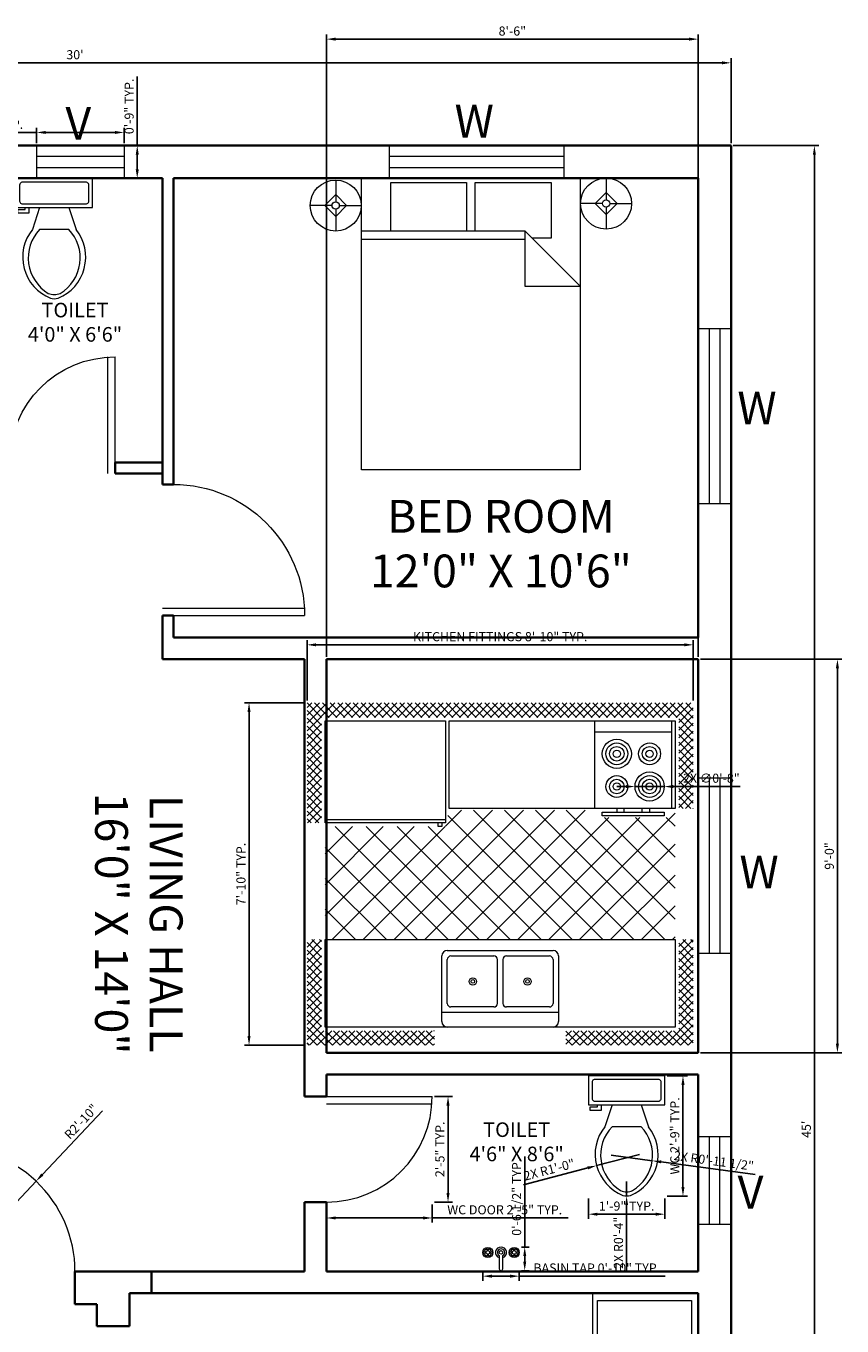
# Model space of a CAD drawing. Units: inches. Extents: x 1642 to 5612, y 1595 to 4064.
# Tile 3 of 6: x 1842 to 2066, y 1811 to 2168. Entities that reach past the tile are written whole.
import ezdxf

# ---------------------------------------------------------------- set-up
doc = ezdxf.new("R2010")
doc.units = ezdxf.units.IN
for name, color, linetype, lineweight in [('A-ANNO-DIMS', 2, 'Continuous', 18), ('A-ANNO-TEXT', 7, 'Continuous', 18), ('A-AREA-IDEN', 7, 'Continuous', 25), ('A-DOOR', 3, 'Continuous', 18), ('A-FLOR-FIXT', 9, 'Continuous', 18), ('A-FURN', 8, 'Continuous', 13), ('A-GLAZ', 4, 'Continuous', 18), ('A-WALL', 7, 'Continuous', 35)]:
    doc.layers.add(name, color=color, linetype=linetype, lineweight=lineweight)
doc.styles.get("Standard").update_dxf_attribs({"font": 'arial.ttf'})
doc.dimstyles.new('ISO-25', dxfattribs={"dimtxt": 2.5, "dimasz": 2.5, "dimexe": 1.25, "dimexo": 0.625, "dimtad": 1, "dimdec": 0, "dimlunit": 3, "dimtxsty": 'Standard', "dimcen": 2.5, "dimadec": 0, "dimazin": 0, "dimtfac": 1, "dimtdec": 0, "dimtmove": 0, "dimatfit": 3, "dimfxl": 1, "dimarcsym": 0})

# ---------------------------------------------------------------- blocks, each defined once
blk = doc.blocks.new('Toilet - top')
for p, q in [((9.5, -6), (9.5, -2)), ((-10, -8.5), (-8, -8.5)), ((-10, -9.5), (-10, -8.5)), ((-7, -9.5), (-10, -9.5)), ((-8, -8.5), (-8, -8)), ((-7, -8), (-7, -9.5)), ((-4, -8), (-6, -14)), ((4, -8), (6, -14)), ((4, -14), (-4, -14))]:
    blk.add_line(p, q)
blk.add_lwpolyline([(10.5, -8), (10.5, 0), (-10.5, 0), (-10.5, -8)], close=True)
for points in [[(-9.5, -2), (-9.5, -6)], [(8.5, -1), (-8.5, -1)], [(-8.5, -7), (8.5, -7)]]:
    blk.add_lwpolyline(points)
for centre, radius, start, end in [((-8.62, -1.88), 0.884, 81.8699, 188.1301), ((8.62, -1.88), 0.884, 351.8699, 98.1301), ((-8.62, -6.12), 0.884, 171.8699, 278.1301), ((8.62, -6.12), 0.884, 261.8699, 8.1301), ((3.52, -21.58), 12.17, 141.4691, 247.9714), ((4.2, -21.82), 11.33, 136.3677, 238.9468), ((-3.52, -21.58), 12.17, 292.0284, 38.5307), ((-4.2, -21.82), 11.33, 301.053, 43.6321), ((0, -27.88), 4, 245.7318, 294.2682), ((0, -29), 4, 254.8605, 285.1395)]:
    blk.add_arc(centre, radius, start, end)
blk = doc.blocks.new('Faucet - Bathroom top')
for p, q in [((-4.107, 0.125), (-4.375, 0.125)), ((-3.75, 0.4788), (-3.75, 0.75)), ((-3.5, 0.482), (-3.5, 0.75)), ((-3.1461, 0.125), (-2.875, 0.125)), ((3.143, 0.125), (2.875, 0.125)), ((3.5, 0.4788), (3.5, 0.75)), ((3.75, 0.482), (3.75, 0.75)), ((4.1039, 0.125), (4.375, 0.125)), ((-4.1039, -0.125), (-4.375, -0.125)), ((-3.75, -0.4821), (-3.75, -0.75)), ((-3.5, -0.4789), (-3.5, -0.75)), ((-3.143, -0.125), (-2.875, -0.125)), ((-0.5, -0.8639), (-0.5, -4.5)), ((0.5, -4.5), (0.5, -0.8631)), ((3.1461, -0.125), (2.875, -0.125)), ((3.5, -0.4821), (3.5, -0.75)), ((3.75, -0.4789), (3.75, -0.75)), ((4.107, -0.125), (4.375, -0.125))]:
    blk.add_line(p, q)
for centre, radius in [((-3.625, 0), 1.375), ((-4.625, 0), 0.2795), ((-3.625, 0), 0.5), ((-3.625, 1), 0.2795), ((-2.625, 0), 0.2795), ((0, 0), 0.5), ((3.625, 0), 1.375), ((2.625, 0), 0.2795), ((3.625, 0), 0.5), ((3.625, 1), 0.2795), ((4.625, 0), 0.2795), ((-3.625, -1), 0.2795), ((3.625, -1), 0.2795)]:
    blk.add_circle(centre, radius)
for centre, radius, start, end in [((-3.625, 0), 1, 105.2407, 164.2093), ((-3.625, 0), 1, 16.44125, 74.07887), ((0, 0), 1.5, 289.6514, 250.3603), ((0, 0), 1, 300.3431, 239.7554), ((3.625, 0), 1, 106.12, 164.0884), ((3.625, 0), 1, 16.23422, 73.90469), ((-3.625, 0), 1, 196.2342, 253.9047), ((-3.625, 0), 1, 286.12, 344.0884), ((3.625, 0), 1, 196.4413, 254.0789), ((3.625, 0), 1, 285.2407, 344.2093), ((0, -4.5), 0.5, 180, 0)]:
    blk.add_arc(centre, radius, start, end)
blk = doc.blocks.new('Kitchen Layout - 7 x 8 ft')
for p, q in [((-5, 81.32), (2.68, 89)), ((-5, 83.44), (0.56, 89)), ((-5, 85.56), (-1.56, 89)), ((-5, 87.68), (-3.68, 89)), ((-1, 84.97), (-5, 88.97)), ((-1, 82.85), (-5, 86.85)), ((1.09, 85), (-2.91, 89)), ((3.21, 85), (-0.79, 89)), ((0.81, 85), (4.81, 89)), ((5.34, 85), (1.34, 89)), ((2.93, 85), (6.93, 89)), ((7.46, 85), (3.46, 89)), ((5.05, 85), (9.05, 89)), ((9.58, 85), (5.58, 89)), ((7.17, 85), (11.17, 89)), ((11.7, 85), (7.7, 89)), ((9.29, 85), (13.29, 89)), ((13.82, 85), (9.82, 89)), ((11.41, 85), (15.41, 89)), ((15.94, 85), (11.94, 89)), ((13.53, 85), (17.53, 89)), ((18.06, 85), (14.06, 89)), ((15.65, 85), (19.65, 89)), ((20.18, 85), (16.18, 89)), ((17.78, 85), (21.78, 89)), ((22.31, 85), (18.31, 89)), ((19.9, 85), (23.9, 89)), ((24.43, 85), (20.43, 89)), ((22.02, 85), (26.02, 89)), ((26.55, 85), (22.55, 89)), ((24.14, 85), (28.14, 89)), ((28.67, 85), (24.67, 89)), ((26.26, 85), (30.26, 89)), ((30.79, 85), (26.79, 89)), ((28.38, 85), (32.38, 89)), ((32.91, 85), (28.91, 89)), ((30.5, 85), (34.5, 89)), ((35.03, 85), (31.03, 89)), ((32.63, 85), (36.63, 89)), ((37.16, 85), (33.16, 89)), ((34.75, 85), (38.75, 89)), ((39.28, 85), (35.28, 89)), ((36.87, 85), (40.87, 89)), ((41.4, 85), (37.4, 89)), ((38.99, 85), (42.99, 89)), ((43.52, 85), (39.52, 89)), ((41.11, 85), (45.11, 89)), ((45.64, 85), (41.64, 89)), ((43.23, 85), (47.23, 89)), ((47.76, 85), (43.76, 89)), ((45.35, 85), (49.35, 89)), ((49.88, 85), (45.88, 89)), ((47.47, 85), (51.47, 89)), ((52, 85), (48, 89)), ((49.6, 85), (53.6, 89)), ((54.13, 85), (50.13, 89)), ((51.72, 85), (55.72, 89)), ((56.25, 85), (52.25, 89)), ((53.84, 85), (57.84, 89)), ((58.37, 85), (54.37, 89)), ((55.96, 85), (59.96, 89)), ((60.49, 85), (56.49, 89)), ((58.08, 85), (62.08, 89)), ((62.61, 85), (58.61, 89)), ((60.2, 85), (64.2, 89)), ((64.73, 85), (60.73, 89)), ((62.32, 85), (66.32, 89)), ((66.85, 85), (62.85, 89)), ((64.45, 85), (68.45, 89)), ((68.97, 85), (64.97, 89)), ((66.57, 85), (70.57, 89)), ((71.1, 85), (67.1, 89)), ((68.69, 85), (72.69, 89)), ((73.22, 85), (69.22, 89)), ((70.81, 85), (74.81, 89)), ((75.34, 85), (71.34, 89)), ((72.93, 85), (76.93, 89)), ((77.46, 85), (73.46, 89)), ((75.05, 85), (79.05, 89)), ((79.58, 85), (75.58, 89)), ((77.17, 85), (81.17, 89)), ((81.7, 85), (77.7, 89)), ((79.29, 85), (83.29, 89)), ((83.82, 85), (79.82, 89)), ((81.42, 85), (85.42, 89)), ((85.95, 85), (81.95, 89)), ((83.54, 85), (87.54, 89)), ((88.07, 85), (84.07, 89)), ((85.66, 85), (89.66, 89)), ((90.19, 85), (86.19, 89)), ((87.78, 85), (91.78, 89)), ((92.31, 85), (88.31, 89)), ((89.9, 85), (93.9, 89)), ((94.43, 85), (90.43, 89)), ((92.02, 85), (96.02, 89)), ((96.55, 85), (92.55, 89)), ((94.14, 85), (98.14, 89)), ((101, 82.67), (94.67, 89)), ((96.27, 85), (100.27, 89)), ((101, 84.79), (96.79, 89)), ((97, 83.61), (101, 87.61)), ((101, 86.92), (98.92, 89)), ((-1, 80.73), (-5, 84.73)), ((-5, 79.19), (-1, 83.19)), ((-1, 78.61), (-5, 82.61)), ((34, 84), (96, 84)), ((34, 60), (34, 84)), ((96, 84), (96, 60)), ((97, 81.49), (101, 85.49)), ((101, 80.55), (97, 84.55)), ((97, 79.37), (101, 83.37)), ((101, 78.43), (97, 82.43)), ((-5, 77.07), (-1, 81.07)), ((-1, 76.49), (-5, 80.49)), ((-5, 74.95), (-1, 78.95)), ((74, 81), (95, 81)), ((97, 77.25), (101, 81.25)), ((101, 76.31), (97, 80.31)), ((97, 75.13), (101, 79.13)), ((-1, 74.36), (-5, 78.36)), ((-5, 72.83), (-1, 76.83)), ((-1, 72.24), (-5, 76.24)), ((101, 74.19), (97, 78.19)), ((97, 73.01), (101, 77.01)), ((101, 72.07), (97, 76.07)), ((-5, 70.71), (-1, 74.71)), ((-1, 70.12), (-5, 74.12)), ((-5, 68.59), (-1, 72.59)), ((-1, 68), (-5, 72)), ((97, 70.89), (101, 74.89)), ((101, 69.95), (97, 73.95)), ((97, 68.76), (101, 72.76)), ((101, 67.82), (97, 71.82)), ((-5, 66.47), (-1, 70.47)), ((-1, 65.88), (-5, 69.88)), ((-5, 64.35), (-1, 68.35)), ((97, 66.64), (101, 70.64)), ((101, 65.7), (97, 69.7)), ((97, 64.52), (101, 68.52)), ((-1, 63.76), (-5, 67.76)), ((-5, 62.22), (-1, 66.22)), ((-1, 61.64), (-5, 65.64)), ((101, 63.58), (97, 67.58)), ((97, 62.4), (101, 66.4)), ((101, 61.46), (97, 65.46)), ((97, 60.28), (101, 64.28)), ((-5, 60.1), (-1, 64.1)), ((-1, 59.52), (-5, 63.52)), ((-5, 57.98), (-1, 61.98)), ((-1, 57.39), (-5, 61.39)), ((100.34, 60), (97, 63.34)), ((98.22, 60), (97, 61.22)), ((98.84, 60), (101, 62.16)), ((-1.73, 56), (-5, 59.27)), ((-3.85, 56), (-5, 57.15)), ((-4.86, 56), (-1, 59.86)), ((-2.74, 56), (-1, 57.74)), ((10.4, 24), (45.9, 59.5)), ((18.88, 24), (54.38, 59.5)), ((27.37, 24), (62.87, 59.5)), ((33.03, 55.11), (37.41, 59.5)), ((67.71, 24), (33.68, 58.04)), ((96, 60), (34, 60)), ((35.85, 24), (71.35, 59.5)), ((76.2, 24), (40.7, 59.5)), ((44.34, 24), (77.84, 57.5)), ((84.68, 24), (49.18, 59.5)), ((52.82, 24), (86.32, 57.5)), ((93.17, 24), (57.67, 59.5)), ((61.31, 24), (96, 58.69)), ((96, 29.65), (66.15, 59.5)), ((96, 38.14), (76.64, 57.5)), ((80, 60), (80, 59)), ((82, 59), (82, 60)), ((96, 46.63), (85.13, 57.5)), ((87, 59), (87, 60)), ((89, 60), (89, 59)), ((96, 55.11), (93.57, 57.54)), ((100.96, 60), (101, 60.04)), ((0, 57), (33, 57)), ((0, 30.57), (24.43, 55)), ((0, 39.06), (15.94, 55)), ((0, 47.54), (7.46, 55)), ((1.91, 24), (32.91, 55)), ((33.77, 24), (2.77, 55)), ((42.26, 24), (11.26, 55)), ((50.74, 24), (19.74, 55)), ((59.23, 24), (28.23, 55)), ((31, 55), (31, 56)), ((32, 55), (31, 55)), ((32, 56), (32, 55)), ((69.79, 24), (96, 50.21)), ((25.29, 24), (0, 49.29)), ((16.8, 24), (0, 40.8)), ((78.28, 24), (96, 41.72)), ((8.32, 24), (0, 32.32)), ((86.76, 24), (96, 33.24)), ((-5, 21.92), (-2.92, 24)), ((-5, 19.8), (-1, 23.8)), ((-1, 19.21), (-5, 23.21)), ((-5, 17.68), (-1, 21.68)), ((-1, 21.33), (-3.67, 24)), ((-1, 23.45), (-1.55, 24)), ((0, 24), (96, 24)), ((0, 0), (0, 24)), ((95.25, 24), (96, 24.75)), ((96, 24), (96, 0)), ((97, 22.1), (98.9, 24)), ((97, 19.97), (101, 23.97)), ((101, 19.03), (97, 23.03)), ((97, 17.85), (101, 21.85)), ((101, 21.16), (98.16, 24)), ((101, 23.28), (100.28, 24)), ((-1, 17.09), (-5, 21.09)), ((-5, 15.55), (-1, 19.55)), ((-1, 14.97), (-5, 18.97)), ((47.25, 6.5), (47.25, 18.5)), ((48.75, 18.5), (48.75, 6.5)), ((101, 16.91), (97, 20.91)), ((97, 15.73), (101, 19.73)), ((101, 14.79), (97, 18.79)), ((-5, 13.43), (-1, 17.43)), ((-1, 12.85), (-5, 16.85)), ((-5, 11.31), (-1, 15.31)), ((-1, 10.73), (-5, 14.73)), ((97, 13.61), (101, 17.61)), ((101, 12.67), (97, 16.67)), ((97, 11.49), (101, 15.49)), ((101, 10.55), (97, 14.55)), ((-5, 9.19), (-1, 13.19)), ((-1, 8.6), (-5, 12.6)), ((-5, 7.07), (-1, 11.07)), ((97, 9.37), (101, 13.37)), ((101, 8.43), (97, 12.43)), ((97, 7.25), (101, 11.25)), ((-1, 6.48), (-5, 10.48)), ((-5, 4.95), (-1, 8.95)), ((-1, 4.36), (-5, 8.36)), ((101, 6.31), (97, 10.31)), ((97, 5.12), (101, 9.12)), ((101, 4.18), (97, 8.18)), ((-5, 2.83), (-1, 6.83)), ((-1, 2.24), (-5, 6.24)), ((-5, 0.71), (-1, 4.71)), ((-1, 0.12), (-5, 4.12)), ((64, 4), (32, 4)), ((97, 3), (101, 7)), ((101, 2.06), (97, 6.06)), ((97, 0.88), (101, 4.88)), ((101, -0.06), (97, 3.94)), ((-5, -1.42), (-1, 2.58)), ((2, -5), (-5, 2)), ((-5, -3.54), (-1, 0.46)), ((96, 0), (0, 0)), ((93.24, -5), (101, 2.76)), ((95.36, -5), (101, 0.64)), ((101, -2.18), (97, 1.82)), ((-0.12, -5), (-5, -0.12)), ((-2.25, -5), (-5, -2.25)), ((-4.34, -5), (-0.34, -1)), ((-2.22, -5), (1.78, -1)), ((-0.1, -5), (3.9, -1)), ((4.12, -5), (0.12, -1)), ((2.02, -5), (6.02, -1)), ((6.24, -5), (2.24, -1)), ((4.14, -5), (8.14, -1)), ((8.36, -5), (4.36, -1)), ((6.27, -5), (10.27, -1)), ((10.48, -5), (6.48, -1)), ((8.39, -5), (12.39, -1)), ((12.6, -5), (8.6, -1)), ((10.51, -5), (14.51, -1)), ((14.73, -5), (10.73, -1)), ((12.63, -5), (16.63, -1)), ((16.85, -5), (12.85, -1)), ((14.75, -5), (18.75, -1)), ((18.97, -5), (14.97, -1)), ((16.87, -5), (20.87, -1)), ((21.09, -5), (17.09, -1)), ((18.99, -5), (22.99, -1)), ((23.21, -5), (19.21, -1)), ((21.11, -5), (25.11, -1)), ((25.33, -5), (21.33, -1)), ((23.24, -5), (27.24, -1)), ((27.45, -5), (23.45, -1)), ((25.36, -5), (29.36, -1)), ((29.57, -5), (25.57, -1)), ((27.48, -5), (30, -2.48)), ((30, -3.3), (27.7, -1)), ((30, -1.18), (29.82, -1)), ((66, -2.54), (67.54, -1)), ((66, -4.66), (69.66, -1)), ((69.88, -5), (66, -1.12)), ((67.76, -5), (66, -3.24)), ((67.78, -5), (71.78, -1)), ((72, -5), (68, -1)), ((69.9, -5), (73.9, -1)), ((74.12, -5), (70.12, -1)), ((72.03, -5), (76.03, -1)), ((76.24, -5), (72.24, -1)), ((74.15, -5), (78.15, -1)), ((78.36, -5), (74.36, -1)), ((76.27, -5), (80.27, -1)), ((80.49, -5), (76.49, -1)), ((78.39, -5), (82.39, -1)), ((82.61, -5), (78.61, -1)), ((80.51, -5), (84.51, -1)), ((84.73, -5), (80.73, -1)), ((82.63, -5), (86.63, -1)), ((86.85, -5), (82.85, -1)), ((84.75, -5), (88.75, -1)), ((88.97, -5), (84.97, -1)), ((86.88, -5), (90.88, -1)), ((91.09, -5), (87.09, -1)), ((89, -5), (93, -1)), ((93.21, -5), (89.21, -1)), ((91.12, -5), (95.12, -1)), ((95.34, -5), (91.34, -1)), ((97.46, -5), (93.46, -1)), ((99.58, -5), (95.58, -1)), ((101, -4.3), (97, -0.3)), ((97.48, -5), (101, -1.48)), ((-4.37, -5), (-5, -4.37)), ((29.6, -5), (30, -4.6)), ((99.6, -5), (101, -3.6))]:
    blk.add_line(p, q)
for points in [[(0, 56), (0, 84), (33, 84), (33, 56)], [(74, 60), (74, 84), (95, 84), (95, 60)], [(76, 58), (76, 59), (93, 59), (93, 58)]]:
    blk.add_lwpolyline(points, close=True)
for points in [[(32, 1.5), (32, 19.5)], [(33.5, 21), (62.5, 21)], [(33.5, 6.5), (33.5, 18.5)], [(34.5, 19.5), (46.25, 19.5)], [(49.75, 19.5), (61.5, 19.5)], [(62.5, 18.5), (62.5, 6.5)], [(64, 19.5), (64, 1.5)], [(46.25, 5.5), (34.5, 5.5)], [(61.5, 5.5), (49.75, 5.5)], [(62.5, 0), (33.5, 0)]]:
    blk.add_lwpolyline(points)
for centre, radius in [((80, 75), 4), ((80, 75), 3), ((80, 75), 2), ((80, 75), 1), ((89, 75), 3), ((89, 75), 2), ((89, 75), 1), ((80, 66), 3), ((80, 66), 2), ((89, 66), 4), ((89, 66), 3), ((89, 66), 2), ((80, 66), 1), ((89, 66), 1), ((40.5, 12.5), 1), ((40.5, 12.5), 0.5), ((55.5, 12.5), 1), ((55.5, 12.5), 0.5)]:
    blk.add_circle(centre, radius)
for centre, radius, start, end in [((33.5, 19.5), 1.5, 90, 180), ((34.5, 18.5), 1, 90, 180), ((46.25, 18.5), 1, 0, 90), ((49.75, 18.5), 1, 90, 180), ((61.5, 18.5), 1, 0, 90), ((62.5, 19.5), 1.5, 0, 90), ((34.5, 6.5), 1, 180, 270), ((46.25, 6.5), 1, 270, 0), ((49.75, 6.5), 1, 180, 270), ((61.5, 6.5), 1, 270, 0), ((33.5, 1.5), 1.5, 180, 270), ((62.5, 1.5), 1.5, 270, 0)]:
    blk.add_arc(centre, radius, start, end)
blk = doc.blocks.new('Bed - Queen')
for p, q in [((0, -80.00003), (0, 0)), ((0, 0), (59.99999, 0)), ((59.99999, 0), (59.99999, -80.00003)), ((7.99999, -1.2), (28.79998, -1.2)), ((7.99999, -14.4), (7.99999, -1.2)), ((28.79998, -1.2), (28.79998, -14.4)), ((31.19999, -1.2), (51.99999, -1.2)), ((31.19999, -14.4), (31.19999, -1.2)), ((51.99999, -1.2), (51.99999, -16.4)), ((0, -14.4), (44.8, -14.4)), ((44.8, -16.8), (0, -16.8)), ((59.99999, -29.6), (44.8, -14.4)), ((44.8, -14.4), (44.8, -29.6)), ((51.99999, -16.4), (46.79936, -16.4)), ((44.8, -29.6), (59.99999, -29.6)), ((59.99999, -80.00003), (0, -80.00003))]:
    blk.add_line(p, q)
blk = doc.blocks.new('Lamp - Table')
for p, q in [((0, 7), (0, 1)), ((-1, 0), (-7, 0)), ((0, 3), (-3, 0)), ((-3, 0), (0, -3)), ((3, 0), (0, 3)), ((0, -3), (3, 0)), ((1, 0), (7, 0)), ((0, -1), (0, -7))]:
    blk.add_line(p, q)
for radius in [7, 1]:
    blk.add_circle((0, 0), radius)
blk = doc.blocks.new('*D10')
at = {"layer": 'A-ANNO-DIMS', "color": 0, "lineweight": -2, "transparency": 16777216}
for p, q in [((1675.28, 2135.62), (1675.28, 2158.94)), ((2035.28, 2135.62), (2035.28, 2158.94)), ((1677.78, 2157.69), (2032.78, 2157.69))]:
    blk.add_line(p, q, dxfattribs=at)
at = {"layer": 'A-ANNO-DIMS', "color": 0, "transparency": 16777216}
for points in [[(1677.78, 2158.1), (1677.78, 2157.27), (1675.28, 2157.69)], [(2032.78, 2158.1), (2032.78, 2157.27), (2035.28, 2157.69)]]:
    blk.add_solid(points, dxfattribs=at)
at = {"layer": 'Defpoints', "color": 0, "transparency": 16777216}
for p in [(2035.28, 2157.69), (1675.28, 2134.99), (2035.28, 2134.99)]:
    blk.add_point(p, dxfattribs=at)
at = {"layer": 'A-ANNO-DIMS', "color": 0, "transparency": 16777216, "insert": (1855.28, 2159.59), "char_height": 2.5, "attachment_point": 5}
blk.add_mtext("30'", dxfattribs=at)
blk = doc.blocks.new('*D11')
at = {"layer": 'A-ANNO-DIMS', "color": 0, "lineweight": -2, "transparency": 16777216}
for p, q in [((2035.91, 2134.99), (2059.41, 2134.99)), ((2058.16, 2132.49), (2058.16, 1597.49)), ((2035.91, 1594.99), (2059.41, 1594.99))]:
    blk.add_line(p, q, dxfattribs=at)
at = {"layer": 'A-ANNO-DIMS', "color": 0, "transparency": 16777216}
for points in [[(2057.74, 2132.49), (2058.57, 2132.49), (2058.16, 2134.99)], [(2057.74, 1597.49), (2058.57, 1597.49), (2058.16, 1594.99)]]:
    blk.add_solid(points, dxfattribs=at)
at = {"layer": 'Defpoints', "color": 0, "transparency": 16777216}
for p in [(2035.28, 2134.99), (2035.28, 1594.99), (2058.16, 1594.99)]:
    blk.add_point(p, dxfattribs=at)
at = {"layer": 'A-ANNO-DIMS', "color": 0, "transparency": 16777216, "insert": (2056.26, 1864.99), "char_height": 2.5, "width": 4.3062, "attachment_point": 5, "rotation": 90}
blk.add_mtext("45'", dxfattribs=at)
blk = doc.blocks.new('WIN-48x9')
for p, q in [((0, 48), (0, 0)), ((9, 48), (0, 48)), ((3, 48), (3, 0)), ((6, 0), (6, 48)), ((9, 0), (9, 48)), ((0, 0), (9, 0))]:
    blk.add_line(p, q)
blk = doc.blocks.new('VENT-24x9')
for p, q in [((9, 24), (0, 24)), ((0, 24), (0, 0)), ((3, 24), (3, 0)), ((6, 0), (6, 24)), ((9, 0), (9, 24)), ((9, 0), (0, 0))]:
    blk.add_line(p, q)
blk = doc.blocks.new('DOOR-SWING-36')
for p, q in [((36, 2), (0, 2)), ((36, 0), (0, 0))]:
    blk.add_line(p, q)
blk.add_arc((36, 0), 36, 90, 180)
blk = doc.blocks.new('DOOR-SWING-29')
for p, q in [((0, 29), (29, 29)), ((0, 27), (29, 27))]:
    blk.add_line(p, q)
blk.add_arc((0, 29), 29, 270, 0)
blk = doc.blocks.new('SEATING-CUSHION-NARROW')
blk.add_lwpolyline([(0, 17.53), (25.79, 17.53), (25.79, 0), (0, 0)], close=True)
blk = doc.blocks.new('*D32')
at = {"layer": 'A-ANNO-DIMS', "color": 0, "lineweight": -2, "transparency": 16777216}
for p, q in [((1844.76, 2138.58), (1815.36, 2138.58)), ((1844.76, 2135.61), (1844.76, 2139.83)), ((1866.26, 2138.58), (1847.26, 2138.58)), ((1868.76, 2135.61), (1868.76, 2139.83))]:
    blk.add_line(p, q, dxfattribs=at)
at = {"layer": 'A-ANNO-DIMS', "color": 0, "transparency": 16777216}
for points in [[(1847.26, 2139), (1847.26, 2138.17), (1844.76, 2138.58)], [(1866.26, 2139), (1866.26, 2138.17), (1868.76, 2138.58)]]:
    blk.add_solid(points, dxfattribs=at)
at = {"layer": 'Defpoints', "color": 0, "transparency": 16777216}
for p in [(1844.76, 2138.58), (1844.76, 2134.98), (1868.76, 2134.98)]:
    blk.add_point(p, dxfattribs=at)
at = {"layer": 'A-ANNO-DIMS', "color": 0, "transparency": 16777216, "insert": (1828.81, 2140.49), "char_height": 2.5, "attachment_point": 5}
blk.add_mtext('VENT 2\'-0" TYP.', dxfattribs=at)
blk = doc.blocks.new('*D33')
at = {"layer": 'A-ANNO-DIMS', "color": 0, "lineweight": -2, "transparency": 16777216}
for p, q in [((1872.36, 2134.98), (1872.36, 2153.97)), ((1869.38, 2134.98), (1873.61, 2134.98)), ((1872.36, 2128.48), (1872.36, 2132.48)), ((1869.38, 2125.98), (1873.61, 2125.98))]:
    blk.add_line(p, q, dxfattribs=at)
at = {"layer": 'A-ANNO-DIMS', "color": 0, "transparency": 16777216}
for points in [[(1871.94, 2132.48), (1872.78, 2132.48), (1872.36, 2134.98)], [(1871.94, 2128.48), (1872.78, 2128.48), (1872.36, 2125.98)]]:
    blk.add_solid(points, dxfattribs=at)
at = {"layer": 'Defpoints', "color": 0, "transparency": 16777216}
for p in [(1868.76, 2134.98), (1872.36, 2134.98), (1868.76, 2125.98)]:
    blk.add_point(p, dxfattribs=at)
at = {"layer": 'A-ANNO-DIMS', "color": 0, "transparency": 16777216, "insert": (1870.46, 2145.73), "char_height": 2.5, "attachment_point": 5, "rotation": 90}
blk.add_mtext('0\'-9" TYP.', dxfattribs=at)
blk = doc.blocks.new('*D40')
at = {"layer": 'A-ANNO-DIMS', "color": 0, "lineweight": -2, "transparency": 16777216}
for p, q in [((2017.77, 1879.68), (2023.35, 1879.68)), ((2022.1, 1849.13), (2022.1, 1877.18)), ((2017.77, 1846.63), (2023.35, 1846.63))]:
    blk.add_line(p, q, dxfattribs=at)
at = {"layer": 'A-ANNO-DIMS', "color": 0, "transparency": 16777216}
for points in [[(2021.68, 1877.18), (2022.52, 1877.18), (2022.1, 1879.68)], [(2021.68, 1849.13), (2022.52, 1849.13), (2022.1, 1846.63)]]:
    blk.add_solid(points, dxfattribs=at)
at = {"layer": 'Defpoints', "color": 0, "transparency": 16777216}
for p in [(2017.14, 1879.68), (2022.1, 1879.68), (2017.14, 1846.63)]:
    blk.add_point(p, dxfattribs=at)
at = {"layer": 'A-ANNO-DIMS', "color": 0, "transparency": 16777216, "insert": (2020.18, 1863.16), "char_height": 2.5, "attachment_point": 5, "rotation": 90}
blk.add_mtext('WC 2\'-9" TYP.', dxfattribs=at)
blk = doc.blocks.new('*D41')
at = {"layer": 'A-ANNO-DIMS', "color": 0, "lineweight": -2, "transparency": 16777216}
for p, q in [((1996.14, 1846.01), (1996.14, 1840.43)), ((2017.14, 1846.01), (2017.14, 1840.43)), ((1998.64, 1841.68), (2014.64, 1841.68))]:
    blk.add_line(p, q, dxfattribs=at)
at = {"layer": 'A-ANNO-DIMS', "color": 0, "transparency": 16777216}
for points in [[(1998.64, 1842.09), (1998.64, 1841.26), (1996.14, 1841.68)], [(2014.64, 1842.09), (2014.64, 1841.26), (2017.14, 1841.68)]]:
    blk.add_solid(points, dxfattribs=at)
at = {"layer": 'Defpoints', "color": 0, "transparency": 16777216}
for p in [(1996.14, 1846.63), (2017.14, 1846.63), (2017.14, 1841.68)]:
    blk.add_point(p, dxfattribs=at)
at = {"layer": 'A-ANNO-DIMS', "color": 0, "transparency": 16777216, "insert": (2006.64, 1843.58), "char_height": 2.5, "attachment_point": 5}
blk.add_mtext('1\'-9" TYP.', dxfattribs=at)
blk = doc.blocks.new('*D42')
at = {"layer": 'A-ANNO-DIMS', "color": 0, "lineweight": -2, "transparency": 16777216}
for p, q in [((1967.18, 1825.54), (1967.18, 1823.42)), ((1969.68, 1824.67), (1974.68, 1824.67)), ((1977.18, 1825.54), (1977.18, 1823.42)), ((1977.18, 1824.67), (2017.22, 1824.67))]:
    blk.add_line(p, q, dxfattribs=at)
at = {"layer": 'A-ANNO-DIMS', "color": 0, "transparency": 16777216}
for points in [[(1969.68, 1825.09), (1969.68, 1824.25), (1967.18, 1824.67)], [(1974.68, 1825.09), (1974.68, 1824.25), (1977.18, 1824.67)]]:
    blk.add_solid(points, dxfattribs=at)
at = {"layer": 'Defpoints', "color": 0, "transparency": 16777216}
for p in [(1967.18, 1826.17), (1977.18, 1826.17), (1977.18, 1824.67)]:
    blk.add_point(p, dxfattribs=at)
at = {"layer": 'A-ANNO-DIMS', "color": 0, "transparency": 16777216, "insert": (1998.45, 1826.59), "char_height": 2.5, "attachment_point": 5}
blk.add_mtext('BASIN TAP 0\'-10" TYP.', dxfattribs=at)
blk = doc.blocks.new('*D43')
at = {"layer": 'A-ANNO-DIMS', "color": 0, "lineweight": -2, "transparency": 16777216}
for p, q in [((1978.68, 1832.67), (1978.68, 1857.48)), ((1977.81, 1832.67), (1979.93, 1832.67)), ((1978.68, 1828.67), (1978.68, 1830.17)), ((1977.81, 1826.17), (1979.93, 1826.17))]:
    blk.add_line(p, q, dxfattribs=at)
at = {"layer": 'A-ANNO-DIMS', "color": 0, "transparency": 16777216}
for points in [[(1978.27, 1830.17), (1979.1, 1830.17), (1978.68, 1832.67)], [(1978.27, 1828.67), (1979.1, 1828.67), (1978.68, 1826.17)]]:
    blk.add_solid(points, dxfattribs=at)
at = {"layer": 'Defpoints', "color": 0, "transparency": 16777216}
for p in [(1977.18, 1832.67), (1978.68, 1832.67), (1977.18, 1826.17)]:
    blk.add_point(p, dxfattribs=at)
at = {"layer": 'A-ANNO-DIMS', "color": 0, "transparency": 16777216, "insert": (1976.77, 1846.33), "char_height": 2.5, "attachment_point": 5, "rotation": 90}
blk.add_mtext('0\'-6 1/2" TYP.', dxfattribs=at)
blk = doc.blocks.new('*D44')
at = {"layer": 'A-ANNO-DIMS', "color": 0, "lineweight": -2, "transparency": 16777216}
for p, q in [((1918.94, 1982.68), (1918.94, 1999.2)), ((2024.94, 1982.68), (2024.94, 1999.2)), ((1921.44, 1997.95), (2022.44, 1997.95))]:
    blk.add_line(p, q, dxfattribs=at)
at = {"layer": 'A-ANNO-DIMS', "color": 0, "transparency": 16777216}
for points in [[(1921.44, 1998.37), (1921.44, 1997.53), (1918.94, 1997.95)], [(2022.44, 1998.37), (2022.44, 1997.53), (2024.94, 1997.95)]]:
    blk.add_solid(points, dxfattribs=at)
at = {"layer": 'Defpoints', "color": 0, "transparency": 16777216}
for p in [(2024.94, 1997.95), (1918.94, 1982.05), (2024.94, 1982.05)]:
    blk.add_point(p, dxfattribs=at)
at = {"layer": 'A-ANNO-DIMS', "color": 0, "transparency": 16777216, "insert": (1971.94, 1999.87), "char_height": 2.5, "attachment_point": 5}
blk.add_mtext('KITCHEN FITTINGS 8\'-10" TYP.', dxfattribs=at)
blk = doc.blocks.new('*D45')
at = {"layer": 'A-ANNO-DIMS', "color": 0, "lineweight": -2, "transparency": 16777216}
for p, q in [((1918.31, 1982.05), (1901.79, 1982.05)), ((1903.04, 1890.55), (1903.04, 1979.55)), ((1918.31, 1888.05), (1901.79, 1888.05))]:
    blk.add_line(p, q, dxfattribs=at)
at = {"layer": 'A-ANNO-DIMS', "color": 0, "transparency": 16777216}
for points in [[(1902.62, 1979.55), (1903.45, 1979.55), (1903.04, 1982.05)], [(1902.62, 1890.55), (1903.45, 1890.55), (1903.04, 1888.05)]]:
    blk.add_solid(points, dxfattribs=at)
at = {"layer": 'Defpoints', "color": 0, "transparency": 16777216}
for p in [(1903.04, 1982.05), (1918.94, 1982.05), (1918.94, 1888.05)]:
    blk.add_point(p, dxfattribs=at)
at = {"layer": 'A-ANNO-DIMS', "color": 0, "transparency": 16777216, "insert": (1901.14, 1935.05), "char_height": 2.5, "attachment_point": 5, "rotation": 90}
blk.add_mtext('7\'-10" TYP.', dxfattribs=at)
blk = doc.blocks.new('*D50')
at = {"layer": 'A-ANNO-DIMS', "color": 0, "lineweight": -2, "transparency": 16777216}
for p, q in [((1924.28, 1844.37), (1924.28, 1839.39)), ((1953.28, 1844.37), (1953.28, 1839.39)), ((1926.78, 1840.64), (1950.78, 1840.64)), ((1953.28, 1840.64), (1990.61, 1840.64))]:
    blk.add_line(p, q, dxfattribs=at)
at = {"layer": 'A-ANNO-DIMS', "color": 0, "transparency": 16777216}
for points in [[(1926.78, 1841.06), (1926.78, 1840.23), (1924.28, 1840.64)], [(1950.78, 1841.06), (1950.78, 1840.23), (1953.28, 1840.64)]]:
    blk.add_solid(points, dxfattribs=at)
at = {"layer": 'Defpoints', "color": 0, "transparency": 16777216}
for p in [(1924.28, 1844.99), (1953.28, 1844.99), (1953.28, 1840.64)]:
    blk.add_point(p, dxfattribs=at)
at = {"layer": 'A-ANNO-DIMS', "color": 0, "transparency": 16777216, "insert": (1973.19, 1842.56), "char_height": 2.5, "attachment_point": 5}
blk.add_mtext('WC DOOR 2\'-5" TYP.', dxfattribs=at)
blk = doc.blocks.new('*D51')
at = {"layer": 'A-ANNO-DIMS', "color": 0, "lineweight": -2, "transparency": 16777216}
for p, q in [((1953.91, 1873.99), (1958.88, 1873.99)), ((1957.63, 1847.49), (1957.63, 1871.49)), ((1953.91, 1844.99), (1958.88, 1844.99))]:
    blk.add_line(p, q, dxfattribs=at)
at = {"layer": 'A-ANNO-DIMS', "color": 0, "transparency": 16777216}
for points in [[(1957.21, 1871.49), (1958.05, 1871.49), (1957.63, 1873.99)], [(1957.21, 1847.49), (1958.05, 1847.49), (1957.63, 1844.99)]]:
    blk.add_solid(points, dxfattribs=at)
at = {"layer": 'Defpoints', "color": 0, "transparency": 16777216}
for p in [(1953.28, 1873.99), (1957.63, 1873.99), (1953.28, 1844.99)]:
    blk.add_point(p, dxfattribs=at)
at = {"layer": 'A-ANNO-DIMS', "color": 0, "transparency": 16777216, "insert": (1955.73, 1859.49), "char_height": 2.5, "attachment_point": 5, "rotation": 90}
blk.add_mtext('2\'-5" TYP.', dxfattribs=at)
blk = doc.blocks.new('*D54')
at = {"layer": 'A-ANNO-DIMS', "color": 0, "lineweight": -2, "transparency": 16777216}
for p, q in [((1924.28, 1994.62), (1924.28, 2165.44)), ((1926.78, 2164.19), (2023.78, 2164.19)), ((2026.28, 1994.62), (2026.28, 2165.44))]:
    blk.add_line(p, q, dxfattribs=at)
at = {"layer": 'A-ANNO-DIMS', "color": 0, "transparency": 16777216}
for points in [[(1926.78, 2164.61), (1926.78, 2163.78), (1924.28, 2164.19)], [(2023.78, 2164.61), (2023.78, 2163.78), (2026.28, 2164.19)]]:
    blk.add_solid(points, dxfattribs=at)
at = {"layer": 'Defpoints', "color": 0, "transparency": 16777216}
for p in [(2026.28, 2164.19), (1924.28, 1993.99), (2026.28, 1993.99)]:
    blk.add_point(p, dxfattribs=at)
at = {"layer": 'A-ANNO-DIMS', "color": 0, "transparency": 16777216, "insert": (1975.28, 2166.09), "char_height": 2.5, "attachment_point": 5}
blk.add_mtext('8\'-6"', dxfattribs=at)
blk = doc.blocks.new('*D55')
at = {"layer": 'A-ANNO-DIMS', "color": 0, "lineweight": -2, "transparency": 16777216}
for p, q in [((2026.91, 1993.99), (2065.73, 1993.99)), ((2064.48, 1888.49), (2064.48, 1991.49)), ((2026.91, 1885.99), (2065.73, 1885.99))]:
    blk.add_line(p, q, dxfattribs=at)
at = {"layer": 'A-ANNO-DIMS', "color": 0, "transparency": 16777216}
for points in [[(2064.06, 1991.49), (2064.9, 1991.49), (2064.48, 1993.99)], [(2064.06, 1888.49), (2064.9, 1888.49), (2064.48, 1885.99)]]:
    blk.add_solid(points, dxfattribs=at)
at = {"layer": 'Defpoints', "color": 0, "transparency": 16777216}
for p in [(2026.28, 1993.99), (2064.48, 1993.99), (2026.28, 1885.99)]:
    blk.add_point(p, dxfattribs=at)
at = {"layer": 'A-ANNO-DIMS', "color": 0, "transparency": 16777216, "insert": (2062.58, 1939.99), "char_height": 2.5, "attachment_point": 5, "rotation": 90}
blk.add_mtext('9\'-0"', dxfattribs=at)
blk = doc.blocks.new('*D66')
at = {"layer": 'A-ANNO-DIMS', "color": 0, "lineweight": -2, "transparency": 16777216}
for p, q in [((1862.79, 1870.03), (1846.32, 1852.55)), ((1821.28, 1825.99), (1844.6, 1850.73))]:
    blk.add_line(p, q, dxfattribs=at)
at = {"layer": 'A-ANNO-DIMS', "color": 0, "transparency": 16777216}
blk.add_solid([(1846.02, 1852.84), (1846.62, 1852.27), (1844.6, 1850.73)], dxfattribs=at)
at = {"layer": 'Defpoints', "color": 0, "transparency": 16777216}
for p in [(1844.6, 1850.73), (1821.28, 1825.99)]:
    blk.add_point(p, dxfattribs=at)
at = {"layer": 'A-ANNO-DIMS', "color": 0, "transparency": 16777216, "insert": (1857.21, 1866.88), "char_height": 2.5, "attachment_point": 5, "rotation": 46.6868}
blk.add_mtext('R2\'-10"', dxfattribs=at)
blk = doc.blocks.new('*D68')
at = {"layer": 'A-ANNO-DIMS', "color": 0, "lineweight": -2, "transparency": 16777216}
for p, q in [((2006.44, 1959.05), (2003.94, 1959.05)), ((2008.94, 1959.05), (2016.94, 1959.05)), ((2037.83, 1959.04), (2019.44, 1959.05))]:
    blk.add_line(p, q, dxfattribs=at)
at = {"layer": 'A-ANNO-DIMS', "color": 0, "transparency": 16777216}
for points in [[(2006.44, 1959.47), (2006.44, 1958.64), (2008.94, 1959.05)], [(2019.44, 1959.47), (2019.44, 1958.63), (2016.94, 1959.05)]]:
    blk.add_solid(points, dxfattribs=at)
at = {"layer": 'Defpoints', "color": 0, "transparency": 16777216}
for p in [(2008.94, 1959.05), (2016.94, 1959.05)]:
    blk.add_point(p, dxfattribs=at)
at = {"layer": 'A-ANNO-DIMS', "color": 0, "transparency": 16777216, "insert": (2029.89, 1961.02), "char_height": 2.5, "attachment_point": 5, "rotation": 359.986}
blk.add_mtext('2X ∅0\'-8"', dxfattribs=at)
blk = doc.blocks.new('*D69')
at = {"layer": 'A-ANNO-DIMS', "color": 0, "lineweight": -2, "transparency": 16777216}
for p, q in [((2010.16, 1858.1), (1998.39, 1855.01)), ((1978.37, 1849.75), (1995.98, 1854.37))]:
    blk.add_line(p, q, dxfattribs=at)
at = {"layer": 'A-ANNO-DIMS', "color": 0, "transparency": 16777216}
blk.add_solid([(1995.87, 1854.77), (1996.08, 1853.97), (1998.39, 1855.01)], dxfattribs=at)
at = {"layer": 'Defpoints', "color": 0, "transparency": 16777216}
for p in [(2010.16, 1858.1), (1998.39, 1855.01)]:
    blk.add_point(p, dxfattribs=at)
at = {"layer": 'A-ANNO-DIMS', "color": 0, "transparency": 16777216, "insert": (1985.48, 1853.58), "char_height": 2.5, "attachment_point": 5, "rotation": 14.7184}
blk.add_mtext('2X R1\'-0"', dxfattribs=at)
blk = doc.blocks.new('*D70')
at = {"layer": 'A-ANNO-DIMS', "color": 0, "lineweight": -2, "transparency": 16777216}
for p, q in [((2002.44, 1857.86), (2013.67, 1856.35)), ((2041.89, 1852.56), (2016.15, 1856.02))]:
    blk.add_line(p, q, dxfattribs=at)
at = {"layer": 'A-ANNO-DIMS', "color": 0, "transparency": 16777216}
blk.add_solid([(2016.2, 1856.43), (2016.09, 1855.61), (2013.67, 1856.35)], dxfattribs=at)
at = {"layer": 'Defpoints', "color": 0, "transparency": 16777216}
for p in [(2002.44, 1857.86), (2013.67, 1856.35)]:
    blk.add_point(p, dxfattribs=at)
at = {"layer": 'A-ANNO-DIMS', "color": 0, "transparency": 16777216, "insert": (2030.51, 1856.02), "char_height": 2.5, "attachment_point": 5, "rotation": 352.3421}
blk.add_mtext('2X R0\'-11 1/2"', dxfattribs=at)
blk = doc.blocks.new('*D71')
at = {"layer": 'A-ANNO-DIMS', "color": 0, "lineweight": -2, "transparency": 16777216}
for p, q in [((2006.64, 1850.68), (2006.64, 1846.68)), ((2006.62, 1825.98), (2006.64, 1844.18))]:
    blk.add_line(p, q, dxfattribs=at)
at = {"layer": 'A-ANNO-DIMS', "color": 0, "transparency": 16777216}
blk.add_solid([(2006.22, 1844.18), (2007.05, 1844.18), (2006.64, 1846.68)], dxfattribs=at)
at = {"layer": 'Defpoints', "color": 0, "transparency": 16777216}
for p in [(2006.64, 1850.68), (2006.64, 1846.68)]:
    blk.add_point(p, dxfattribs=at)
at = {"layer": 'A-ANNO-DIMS', "color": 0, "transparency": 16777216, "insert": (2004.73, 1833.83), "char_height": 2.5, "attachment_point": 5, "rotation": 89.9534}
blk.add_mtext('2X R0\'-4"', dxfattribs=at)

msp = doc.modelspace()

# ---------------------------------------------------------------- linework, layer by layer
at = {"layer": 'A-DOOR'}
for p, q in [((1864.28, 2044.99), (1864.28, 2047.99)), ((1879.28, 2007.99), (1882.28, 2007.99))]:
    msp.add_line(p, q, dxfattribs=at)
msp.add_arc((1821.28, 1825.99), 34, 360, 93.3723, dxfattribs=at)
at = {"layer": 'A-FURN'}
msp.add_line((1997.28, 1819.99), (1997.28, 1689.99), dxfattribs=at)
at = {"layer": 'A-WALL'}
for p, q in [((1675.28, 2134.99), (2035.28, 2134.99)), ((2035.28, 2134.99), (2035.28, 1594.99)), ((1831.28, 2125.99), (1879.28, 2125.99)), ((1879.28, 2125.99), (1879.28, 2041.99)), ((1882.28, 2125.99), (1882.28, 2041.99)), ((1882.28, 2125.99), (2026.28, 2125.99)), ((2026.28, 2125.99), (2026.28, 1999.99)), ((1866.28, 2047.99), (1866.28, 2044.99)), ((1866.28, 2044.99), (1866.28, 2047.99)), ((1866.28, 2047.99), (1879.28, 2047.99)), ((1866.28, 2044.99), (1879.28, 2044.99)), ((1879.28, 2041.99), (1882.28, 2041.99)), ((1879.28, 1999.99), (1879.28, 2005.99)), ((1879.28, 2005.99), (1882.28, 2005.99)), ((1879.28, 2005.99), (1879.28, 1999.99)), ((1882.28, 2005.99), (1882.28, 1999.99)), ((1879.28, 1999.99), (1879.28, 1993.99)), ((1882.28, 1999.99), (2026.28, 1999.99)), ((1879.28, 1993.99), (1918.28, 1993.99)), ((1918.28, 1993.99), (1918.28, 1873.99)), ((1924.28, 1993.99), (1924.28, 1885.99)), ((1924.28, 1993.99), (2026.28, 1993.99)), ((2026.28, 1993.99), (2026.28, 1885.99)), ((1924.28, 1885.99), (2026.28, 1885.99)), ((1924.28, 1879.99), (2026.28, 1879.99)), ((1924.28, 1879.99), (1924.28, 1873.99)), ((1924.28, 1879.99), (1924.28, 1873.99)), ((2026.28, 1879.99), (2026.28, 1825.99)), ((1924.28, 1873.99), (1918.28, 1873.99)), ((1918.28, 1844.99), (1924.28, 1844.99)), ((1918.28, 1844.99), (1918.28, 1825.99)), ((1924.28, 1844.99), (1924.28, 1825.99)), ((1855.28, 1816.99), (1855.28, 1825.99)), ((1855.28, 1825.99), (1876.28, 1825.99)), ((1876.28, 1819.99), (1876.28, 1825.99)), ((1912.28, 1825.99), (1876.28, 1825.99)), ((1918.28, 1825.99), (1912.28, 1825.99)), ((1912.28, 1825.99), (1918.28, 1825.99)), ((1924.28, 1825.99), (2026.28, 1825.99)), ((1870.28, 1819.99), (1870.28, 1810.99)), ((1870.28, 1819.99), (1876.28, 1819.99)), ((1876.28, 1819.99), (1912.28, 1819.99)), ((1912.28, 1819.99), (2026.28, 1819.99)), ((2026.28, 1819.99), (2026.28, 1660.99)), ((1861.28, 1816.99), (1855.28, 1816.99)), ((1861.28, 1816.99), (1855.28, 1816.99)), ((1855.28, 1816.99), (1861.28, 1816.99)), ((1861.28, 1816.99), (1861.28, 1810.99)), ((1861.28, 1816.99), (1861.28, 1810.99)), ((1861.28, 1810.99), (1870.28, 1810.99))]:
    msp.add_line(p, q, dxfattribs=at)

# ---------------------------------------------------------------- block references
at = {"layer": 'A-DOOR', "extrusion": (0, 0, -1), "zscale": -1, "rotation": 89.9999999999989}
msp.add_blockref('DOOR-SWING-29', (-1837.28, 2047.99), dxfattribs=at)
at = {"layer": 'A-DOOR', "extrusion": (0, 0, -1), "zscale": -1}
msp.add_blockref('DOOR-SWING-36', (-1918.28, 2005.99), dxfattribs=at)
at = {"layer": 'A-DOOR'}
msp.add_blockref('DOOR-SWING-29', (1924.28, 1844.99), dxfattribs=at)
at = {"layer": 'A-FLOR-FIXT'}
for name, p in [('Toilet - top', (1849.58, 2125.95)), ('Kitchen Layout - 7 x 8 ft', (1923.94, 1893.05)), ('Toilet - top', (2006.64, 1879.68)), ('Faucet - Bathroom top', (1972.18, 1831.17))]:
    msp.add_blockref(name, p, dxfattribs=at)
at = {"layer": 'A-FURN'}
for name, p in [('Lamp - Table', (1926.81, 2118.53)), ('Bed - Queen', (1933.92, 2126.01)), ('Lamp - Table', (2001, 2119.06)), ('SEATING-CUSHION-NARROW', (1998.68, 1800.43))]:
    msp.add_blockref(name, p, dxfattribs=at)
at = {"layer": 'A-GLAZ'}
for name, p, rotation in [('VENT-24x9', (1868.76, 2125.98), 90.00000000000072), ('WIN-48x9', (1941.51, 2134.99), 269.9999999999997)]:
    msp.add_blockref(name, p, dxfattribs=dict(at, rotation=rotation))
for name, p in [('WIN-48x9', (2026.28, 2036.72)), ('WIN-48x9', (2026.28, 1913.32)), ('VENT-24x9', (2026.25, 1838.89))]:
    msp.add_blockref(name, p, dxfattribs=at)

# ---------------------------------------------------------------- texts
at = {"layer": 'A-ANNO-TEXT', "char_height": 9, "attachment_point": 1}
for s, width, insert in [('\\pxqc;V', 37.3133, (1837.52, 2145.59)), ('\\pxqc;W', 122.7897, (1903.43, 2146.19)), ('\\pxqc;W', 122.7897, (1981.02, 2067.47)), ('\\pxqc;W', 122.7897, (1981.59, 1940.09)), ('\\pxqc;V', 37.3133, (2021.98, 1852.21))]:
    msp.add_mtext_dynamic_manual_height_columns(s, width=width, gutter_width=12.5, heights=[0], dxfattribs=dict(at, insert=insert))
at = {"layer": 'A-AREA-IDEN', "attachment_point": 1}
for s, width, insert, char_height in [('\\pxqc;TOILET\\P4\'0" X 6\'6"', 48, (1831.28, 2091.83), 4), ('\\pxqc;BED ROOM \\P12\'0" X 10\'6"', 95.4247, (1924.43, 2037.73), 9), ('\\pxqc;TOILET \\P4\'6" X 8\'6"', 41.2301, (1955.85, 1866.88), 4)]:
    msp.add_mtext_dynamic_manual_height_columns(s, width=width, gutter_width=12.5, heights=[0], dxfattribs=dict(at, insert=insert, char_height=char_height))
at = {"layer": 'A-AREA-IDEN', "insert": (1884.81, 1967.27), "char_height": 9, "attachment_point": 1, "rotation": 270}
msp.add_mtext_dynamic_manual_height_columns('\\pxqc;LIVING HALL\\P16\'0" X 14\'0"', width=91.6716, gutter_width=12.5, heights=[0], dxfattribs=at)

# ---------------------------------------------------------------- dimensions: what is measured, and where the dimension line sits
at = {"layer": 'A-ANNO-DIMS'}
for base, p1, p2, override, picture, middle in [((2026.28, 2164.19), (1924.28, 1993.99), (2026.28, 1993.99), {"dimdec": 1, "dimlfac": 1, "dimrnd": 0, "dimzin": 1, "dimdsep": 46, "dimlunit": 4, "dimfrac": 2}, '*D54', (1975.28, 2166.09)), ((2035.28, 2157.69), (1675.28, 2134.99), (2035.28, 2134.99), {"dimclrd": 0, "dimclre": 0, "dimclrt": 0}, '*D10', (1855.28, 2159.59))]:
    dim = msp.add_linear_dim(base=base, p1=p1, p2=p2, dimstyle='ISO-25', override=override, dxfattribs=at)
    dim.commit()
    dim.dimension.update_dxf_attribs({"geometry": picture, "text_midpoint": middle})
for base, p1, p2, angle, text, picture, middle in [((1872.36, 2134.98), (1868.76, 2125.98), (1868.76, 2134.98), 90, '<> TYP.', '*D33', (1870.46, 2145.73)), ((1844.76, 2138.58), (1868.76, 2134.98), (1844.76, 2134.98), 180, 'VENT <> TYP.', '*D32', (1828.81, 2140.49)), ((1903.04, 1982.05), (1918.94, 1888.05), (1918.94, 1982.05), 90, '<> TYP.', '*D45', (1901.14, 1935.05)), ((2022.1002, 1879.6793), (2017.1432, 1846.633), (2017.1432, 1879.6793), 90, 'WC <> TYP.', '*D40', (2020.1825, 1863.1562)), ((1957.63, 1873.99), (1953.28, 1844.99), (1953.28, 1873.99), 90, '<> TYP.', '*D51', (1955.73, 1859.49)), ((1978.68, 1832.67), (1977.18, 1826.17), (1977.18, 1832.67), 90, '<> TYP.', '*D43', (1976.77, 1846.33))]:
    dim = msp.add_linear_dim(base=base, p1=p1, p2=p2, angle=angle, text=text, dimstyle='ISO-25', override={"dimdec": 1, "dimlfac": 1, "dimrnd": 0, "dimzin": 1, "dimdsep": 46, "dimlunit": 4, "dimfrac": 2}, dxfattribs=at)
    dim.commit()
    dim.dimension.update_dxf_attribs({"geometry": picture, "text_midpoint": middle})
for base, p1, p2, override, picture, middle in [((2058.16, 1594.99), (2035.28, 2134.99), (2035.28, 1594.99), {"dimclrd": 0, "dimclre": 0, "dimclrt": 0}, '*D11', (2056.26, 1864.99)), ((2064.48, 1993.99), (2026.28, 1885.99), (2026.28, 1993.99), {"dimdec": 1, "dimlfac": 1, "dimrnd": 0, "dimzin": 1, "dimdsep": 46, "dimlunit": 4, "dimfrac": 2}, '*D55', (2062.58, 1939.99))]:
    dim = msp.add_linear_dim(base=base, p1=p1, p2=p2, angle=90, dimstyle='ISO-25', override=override, dxfattribs=at)
    dim.commit()
    dim.dimension.update_dxf_attribs({"geometry": picture, "text_midpoint": middle})
for base, p1, p2, text, picture, middle in [((2024.94, 1997.95), (1918.94, 1982.05), (2024.94, 1982.05), 'KITCHEN FITTINGS <> TYP.', '*D44', (1971.94, 1999.87)), ((1953.28, 1840.64), (1924.28, 1844.99), (1953.28, 1844.99), 'WC DOOR <> TYP.', '*D50', (1973.19, 1842.56)), ((2017.14, 1841.68), (1996.14, 1846.63), (2017.14, 1846.63), '<> TYP.', '*D41', (2006.64, 1843.58)), ((1977.18, 1824.67), (1967.18, 1826.17), (1977.18, 1826.17), 'BASIN TAP <> TYP.', '*D42', (1998.45, 1826.59))]:
    dim = msp.add_linear_dim(base=base, p1=p1, p2=p2, text=text, dimstyle='ISO-25', override={"dimdec": 1, "dimlfac": 1, "dimrnd": 0, "dimzin": 1, "dimdsep": 46, "dimlunit": 4, "dimfrac": 2}, dxfattribs=at)
    dim.commit()
    dim.dimension.update_dxf_attribs({"geometry": picture, "text_midpoint": middle})
dim = msp.add_diameter_dim_2p(p1=(2008.94, 1959.05), p2=(2016.94, 1959.05), text='2X <>', dimstyle='ISO-25', override={"dimdec": 1, "dimlfac": 1, "dimrnd": 0, "dimzin": 1, "dimdsep": 46, "dimlunit": 4, "dimfrac": 2}, dxfattribs=at)
dim.commit()
dim.dimension.update_dxf_attribs({"geometry": '*D68', "text_midpoint": (2029.89, 1959.05), "dimtype": 163})
dim = msp.add_radius_dim(center=(1821.28, 1825.99), mpoint=(1844.6, 1850.73), dimstyle='ISO-25', override={"dimdec": 1, "dimlfac": 1, "dimrnd": 0, "dimzin": 1, "dimdsep": 46, "dimlunit": 4, "dimfrac": 2}, dxfattribs=at)
dim.commit()
dim.dimension.update_dxf_attribs({"geometry": '*D66', "text_midpoint": (1858.6, 1865.58), "dimtype": 164})
for center, mpoint, picture, middle in [((2002.44, 1857.86), (2013.67, 1856.35), '*D70', (2030.51, 1856.02)), ((2010.16, 1858.1), (1998.39, 1855.01), '*D69', (1985.48, 1853.58)), ((2006.64, 1850.68), (2006.64, 1846.68), '*D71', (2004.73, 1833.83))]:
    dim = msp.add_radius_dim(center=center, mpoint=mpoint, text='2X <>', dimstyle='ISO-25', override={"dimdec": 1, "dimlfac": 1, "dimrnd": 0, "dimzin": 1, "dimdsep": 46, "dimlunit": 4, "dimfrac": 2}, dxfattribs=at)
    dim.commit()
    dim.dimension.update_dxf_attribs({"geometry": picture, "text_midpoint": middle})

doc.saveas('drawing.dxf')
